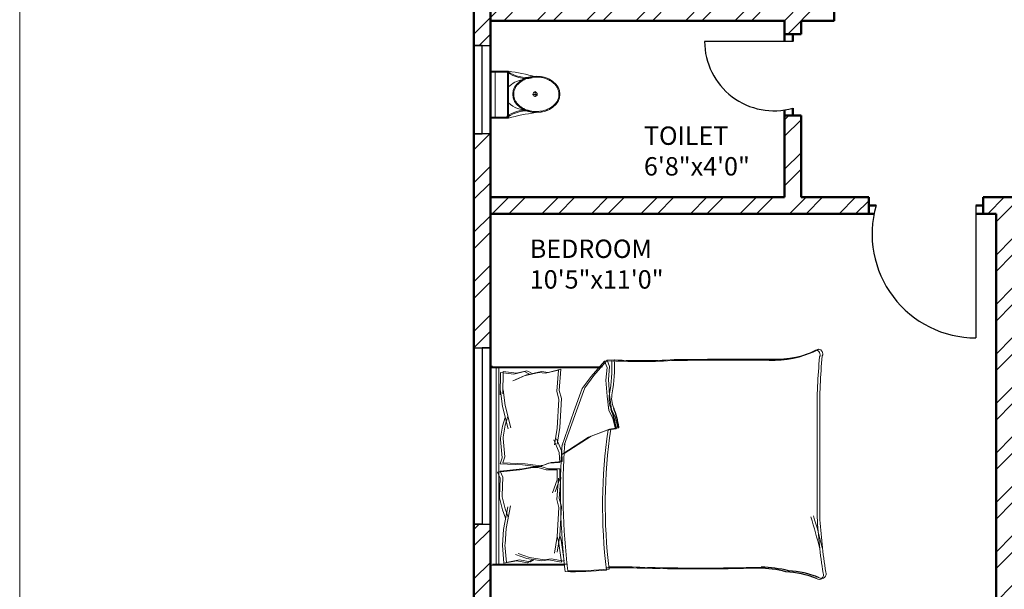
# Model space of a CAD drawing. Units: inches. Extents: x 1901 to 2863, y 888 to 2433.
# Tile 50 of 91: x 1901 to 2169, y 1847 to 2002. Entities that reach past the tile are written whole.
import ezdxf

# ---------------------------------------------------------------- set-up
doc = ezdxf.new("R2010")
doc.units = ezdxf.units.IN
for name, color, linetype, lineweight in [('A-AREA-IDEN', 7, 'Continuous', 18), ('A-DOOR', 4, 'Continuous', 25), ('A-FLOR-FIXT', 9, 'Continuous', 18), ('A-FURN', 8, 'Continuous', 18), ('A-GLAZ', 3, 'Continuous', 25), ('A-WALL', 7, 'Continuous', 50), ('A-WALL-PATT', 8, 'Continuous', 13)]:
    doc.layers.add(name, color=color, linetype=linetype, lineweight=lineweight)
doc.styles.get("Standard").update_dxf_attribs({"font": 'arial.ttf'})

# ---------------------------------------------------------------- blocks, each defined once
blk = doc.blocks.new('A$C31115884')
for p, q in [((283, 498), (223, 498)), ((258, 466), (258, 523)), ((0, 200), (0, 0)), ((520, 200), (0, 200)), ((10, 190), (10, 10)), ((510, 190), (10, 190)), ((510, 10), (510, 190)), ((520, 0), (520, 200)), ((510, 54), (0, 54)), ((10, 10), (510, 10)), ((0, 0), (520, 0))]:
    blk.add_line(p, q)
blk.add_circle((256, 496), 23.6)
for centre, radius, start, end in [((2778, -205), 2807, 165.4549, 171.7133), ((-295, 403), 365, 324.2091, 9.3499), ((-295, 403), 375, 324.2091, 9.3499), ((806, 403), 365, 170.6501, 215.7909), ((3237, 905), 2807, 188.2867, 194.5451), ((384, 406), 293, 190.2774, 224.1564), ((139, 406), 293, 315.8436, 2.6563), ((806, 403), 375, 179.2036, 215.7909)]:
    blk.add_arc(centre, radius, start, end)
blk.add_ellipse((256, 510), major_axis=(0, -261), ratio=0.772727)
blk.add_open_spline([(256, 259), (263, 259), (270, 260), (288, 262), (299, 265), (320, 273), (330, 278), (350, 291), (360, 299), (378, 316), (386, 326), (402, 347), (409, 358), (421, 383), (427, 395), (436, 422), (440, 436), (445, 465), (447, 480), (448, 509), (448, 524), (445, 553), (443, 568), (436, 596), (432, 610), (422, 636), (416, 649), (402, 672), (395, 683), (379, 703), (370, 712), (351, 728), (341, 735), (321, 746), (310, 751), (289, 757), (278, 759), (256, 761), (245, 761), (223, 757), (212, 754), (191, 746), (181, 741), (161, 728), (151, 720), (133, 703), (125, 693), (110, 672), (103, 660), (90, 636), (85, 623), (76, 596), (72, 582), (67, 553), (66, 538), (64, 509), (65, 494), (68, 465), (70, 450), (77, 422), (81, 408), (91, 382), (97, 370), (111, 346), (118, 335), (135, 316), (144, 307), (162, 291), (172, 284), (193, 273), (203, 269), (225, 262), (236, 260), (250, 259), (253, 259), (256, 259)], degree=3, knots=[0, 0, 0, 0, 0.110105, 0.110105, 0.285049, 0.285049, 0.459994, 0.459994, 0.634938, 0.634938, 0.809882, 0.809882, 0.984827, 0.984827, 1.159771, 1.159771, 1.334715, 1.334715, 1.50966, 1.50966, 1.684604, 1.684604, 1.859549, 1.859549, 2.034493, 2.034493, 2.209437, 2.209437, 2.384382, 2.384382, 2.559326, 2.559326, 2.73427, 2.73427, 2.909215, 2.909215, 3.084159, 3.084159, 3.259103, 3.259103, 3.434048, 3.434048, 3.608992, 3.608992, 3.783936, 3.783936, 3.958881, 3.958881, 4.133825, 4.133825, 4.30877, 4.30877, 4.483714, 4.483714, 4.658658, 4.658658, 4.833603, 4.833603, 5.008547, 5.008547, 5.183491, 5.183491, 5.358436, 5.358436, 5.53338, 5.53338, 5.708324, 5.708324, 5.883269, 5.883269, 6.058213, 6.058213, 6.233158, 6.233158, 6.283185, 6.283185, 6.283185, 6.283185])
blk = doc.blocks.new('WIN-48')
for p, q in [((0, 2.25), (0, 4.5)), ((0, 4.5), (0, 0)), ((48, 4.5), (48, 0)), ((48, 2.25), (0, 2.25)), ((48, 0), (48, 2.25))]:
    blk.add_line(p, q)
blk = doc.blocks.new('WIN-24-3')
for p, q in [((0, 0), (0, 4.5)), ((0, 4.5), (0, 2.25)), ((24, 2.25), (24, 4.5)), ((24, 4.5), (24, 0)), ((0, 2.25), (24, 2.25))]:
    blk.add_line(p, q)
blk = doc.blocks.new('DOOR-28')
blk.add_line((28.27, 35.98), (28.27, -0.02))
blk.add_arc((28.27, 28.24), 28.25, 164.0861, 270)

msp = doc.modelspace()

# ---------------------------------------------------------------- hatches: boundary and pattern name
at = {"layer": 'A-WALL-PATT'}
h = msp.add_hatch(dxfattribs=at)
h.set_pattern_fill('ANSI32', color=256)
h.paths.add_polyline_path([(2192.5, 2274.13), (2141.26, 2274.13), (2141.26, 2269.63), (2192.5, 2269.63)])
h.paths.add_polyline_path([(2259.93, 2274.13), (2216.5, 2274.13), (2216.5, 2269.63), (2255.43, 2269.63), (2255.43, 2214.63), (2250.81, 2214.63), (2250.81, 2210.13), (2259.93, 2210.13), (2259.93, 2215.13), (2271.76, 2215.13), (2271.76, 2217.38), (2271.76, 2219.63), (2259.93, 2219.63)])
h.paths.add_polyline_path([(2171.43, 2269.63), (2166.93, 2269.63), (2166.93, 2219.63), (2121.24, 2219.63), (2121.24, 2215.13), (2166.93, 2215.13), (2166.93, 2083.13), (2161.81, 2083.13), (2161.81, 2078.63), (2171.43, 2078.63), (2177, 2078.63), (2177, 2080.88), (2177, 2083.13), (2171.43, 2083.13), (2171.43, 2210.13), (2230.91, 2210.13), (2230.91, 2212.38), (2230.91, 2214.63), (2171.43, 2214.63)])
h.paths.add_polyline_path([(2117.26, 2274.13), (2089.43, 2274.13), (2089.43, 2219.63), (2081.14, 2219.63), (2081.14, 2215.13), (2089.43, 2215.13), (2098, 2215.13), (2098, 2217.38), (2098, 2219.63), (2093.93, 2219.63), (2093.93, 2269.63), (2117.26, 2269.63), (2117.26, 2271.88)])
h.paths.add_polyline_path([(2343.43, 2219.63), (2329.29, 2219.63), (2329.29, 2215.13), (2338.93, 2215.13), (2338.93, 2184.74), (2343.43, 2184.74)])
h.paths.add_polyline_path([(2338.93, 2083.13), (2329.29, 2083.13), (2208.97, 2083.13), (2208.97, 2078.63), (2338.93, 2078.63)])
h.paths.add_polyline_path([(2343.43, 2136.74), (2338.93, 2136.74), (2338.93, 1872.63), (2343.43, 1872.63)])
h.paths.add_polyline_path([(2343.43, 1863.63), (2397.68, 1863.63), (2397.68, 1821.63), (2384.14, 1821.63), (2384.14, 1812.63), (2418.33, 1812.63), (2418.33, 1817.13), (2418.33, 1821.63), (2406.68, 1821.63), (2406.68, 1863.63), (2459.5, 1863.63), (2459.5, 1821.63), (2447.14, 1821.63), (2447.14, 1812.63), (2459.5, 1812.63), (2468.5, 1812.63), (2468.5, 1872.63), (2394.43, 1872.63), (2334.43, 1872.63), (2334.43, 1812.63), (2343.43, 1812.63), (2353.25, 1812.63), (2353.25, 1821.63), (2343.43, 1821.63)])
h.paths.add_polyline_path([(2510.01, 1872.63), (2468.5, 1872.63), (2468.5, 1868.13), (2510.01, 1868.13)])
h.paths.add_polyline_path([(2514.01, 1817.13), (2468.5, 1817.13), (2468.5, 1812.63), (2482.11, 1812.63), (2482.11, 1800.61), (2486.61, 1800.61), (2486.61, 1812.63), (2514.01, 1812.63)])
h.paths.add_polyline_path([(2299.25, 1814.88), (2299.25, 1817.13), (2295.93, 1817.13), (2295.93, 1854.17), (2293.68, 1854.17), (2291.43, 1854.17), (2291.43, 1817.13), (2266.11, 1817.13), (2266.11, 1812.63), (2299.25, 1812.63)])
h.paths.add_polyline_path([(2218.11, 1817.13), (2206.46, 1817.13), (2171.43, 1817.13), (2171.43, 1949.13), (2190.1, 1949.13), (2190.1, 1953.63), (2163.47, 1953.63), (2163.47, 1949.13), (2166.93, 1949.13), (2166.93, 1817.13), (2114.3, 1817.13), (2114.3, 1812.63), (2218.11, 1812.63)])
h.paths.add_polyline_path([(2029.43, 1970.92), (2024.93, 1970.92), (2024.93, 1912.72), (2029.43, 1912.72)])
h.paths.add_polyline_path([(2132.3, 1953.63), (2113.93, 1953.63), (2113.93, 1975.89), (2111.68, 1975.89), (2109.43, 1975.89), (2109.43, 1953.63), (2029.43, 1953.63), (2029.43, 1949.13), (2132.3, 1949.13)])
h.paths.add_polyline_path([(2029.43, 1853.61), (2029.31, 1853.61), (2029.31, 1853.61), (2029.43, 1853.61), (2029.43, 1864.72), (2024.93, 1864.72), (2024.93, 1812.63), (2066.3, 1812.63), (2066.3, 1814.88), (2066.3, 1817.13), (2029.43, 1817.13)])
h.paths.add_polyline_path([(2122.93, 2010.09), (2120.68, 2010.09), (2118.43, 2010.09), (2118.43, 2006.13), (2029.43, 2006.13), (2029.43, 2001.63), (2109.43, 2001.63), (2109.43, 1998.04), (2113.93, 1998.04), (2113.93, 2001.63), (2122.93, 2001.63)])
h.paths.add_polyline_path([(2029.43, 2031.38), (2024.93, 2031.38), (2024.93, 1994.92), (2027.18, 1994.92), (2029.43, 1994.92)])
h.paths.add_polyline_path([(2029.43, 2136.74), (2024.93, 2136.74), (2024.93, 2067.38), (2027.18, 2067.38), (2029.43, 2067.38)])
h.paths.add_polyline_path([(2125.62, 2083.13), (2029.43, 2083.13), (2029.43, 2078.63), (2118.43, 2078.63), (2118.43, 2030.71), (2122.93, 2030.71), (2122.93, 2078.63), (2125.62, 2078.63)])
h.paths.add_polyline_path([(2029.43, 2215.13), (2040.47, 2215.13), (2040.47, 2217.38), (2040.47, 2219.63), (2024.93, 2219.63), (2024.93, 2184.74), (2029.43, 2184.74), (2029.43, 2187.78)])
h.paths.add_polyline_path([(2686.43, 2274.13), (2659.28, 2274.13), (2659.28, 2269.63), (2681.93, 2269.63), (2681.93, 2219.63), (2676.82, 2219.63), (2676.82, 2215.13), (2681.93, 2215.13), (2697.01, 2215.13), (2697.01, 2217.38), (2697.01, 2219.63), (2686.43, 2219.63)])
h.paths.add_polyline_path([(2609.93, 2269.63), (2635.28, 2269.63), (2635.28, 2274.13), (2571.43, 2274.13), (2571.43, 2269.63), (2605.43, 2269.63), (2605.43, 2214.63), (2549.1, 2214.63), (2549.1, 2210.13), (2605.43, 2210.13), (2605.43, 2083.13), (2601.01, 2083.13), (2601.01, 2080.88), (2601.01, 2078.63), (2609.93, 2078.63), (2616.16, 2078.63), (2616.16, 2080.88), (2616.16, 2083.13), (2609.93, 2083.13), (2609.93, 2215.13), (2651.46, 2215.13), (2651.46, 2217.38), (2651.46, 2219.63), (2609.93, 2219.63)])
h.paths.add_polyline_path([(2521.43, 2269.63), (2547.43, 2269.63), (2547.43, 2271.88), (2547.43, 2274.13), (2516.93, 2274.13), (2516.93, 2219.63), (2506.41, 2219.63), (2506.41, 2215.13), (2516.93, 2215.13), (2516.93, 2210.13), (2525.4, 2210.13), (2525.4, 2212.38), (2525.4, 2214.63), (2521.43, 2214.63)])
h.paths.add_polyline_path([(2456.01, 2219.63), (2439.43, 2219.63), (2439.43, 2187.89), (2443.93, 2187.89), (2443.93, 2215.13), (2456.01, 2215.13)])
h.paths.add_polyline_path([(2752.93, 2219.63), (2739.48, 2219.63), (2739.48, 2215.13), (2748.43, 2215.13), (2748.43, 2187.89), (2752.93, 2187.89)])
h.paths.add_polyline_path([(2752.93, 2139.89), (2748.43, 2139.89), (2748.43, 2083.13), (2648.42, 2083.13), (2648.42, 2078.63), (2654.93, 2078.63), (2654.93, 2039.44), (2659.43, 2039.44), (2659.43, 2078.63), (2748.43, 2078.63), (2748.43, 2063.43), (2752.93, 2063.43)])
h.paths.add_polyline_path([(2752.93, 2010.63), (2659.43, 2010.63), (2659.43, 2015.65), (2654.93, 2015.65), (2654.93, 2010.63), (2605.43, 2010.63), (2605.43, 1920.97), (2609.93, 1920.97), (2609.93, 2006.13), (2748.43, 2006.13), (2748.43, 1982.47), (2752.93, 1982.47)])
h.paths.add_polyline_path([(2752.93, 2027.43), (2748.43, 2027.43), (2748.43, 2010.63), (2752.93, 2010.63)])
h.paths.add_polyline_path([(2748.43, 1886.13), (2609.93, 1886.13), (2609.93, 1889.72), (2605.43, 1889.72), (2605.43, 1861.26), (2609.93, 1861.26), (2609.93, 1881.63), (2748.43, 1881.63)])
h.paths.add_polyline_path([(2456.86, 2228.83), (2498.4, 2228.83), (2498.4, 2247.49), (2456.86, 2247.49)], flags=9)
h.paths.add_polyline_path([(2038.6, 2237.42), (2080.17, 2237.42), (2080.17, 2256.08), (2038.6, 2256.08)], flags=9)
h.paths.add_polyline_path([(2292.01, 1062.39), (2539.93, 1062.39), (2539.93, 1099.49), (2292.01, 1099.49)], flags=9)
h.paths.add_polyline_path([(2424.91, 1832.25), (2448.51, 1832.25), (2448.51, 1846.68), (2424.91, 1846.68)], flags=25)
h.paths.add_polyline_path([(2359.08, 1832.25), (2382.68, 1832.25), (2382.68, 1846.68), (2359.08, 1846.68)], flags=25)
h.paths.add_polyline_path([(2352.9, 1684.8), (2367.54, 1684.8), (2367.54, 1697.17), (2352.9, 1697.17)], flags=9)
h.paths.add_polyline_path([(2079.29, 1755.83), (2169.02, 1755.83), (2169.02, 1774.37), (2079.29, 1774.37)], flags=9)
h.paths.add_polyline_path([(2404.09, 1373.86), (2404.09, 1463.59), (2385.54, 1463.59), (2385.54, 1373.86)], flags=9)
h.paths.add_polyline_path([(2268.09, 2236.37), (2309.64, 2236.37), (2309.64, 2255.03), (2268.09, 2255.03)], flags=9)
h.paths.add_polyline_path([(2575.96, 1700.95), (2665.7, 1700.95), (2665.7, 1719.5), (2575.96, 1719.5)], flags=9)
h.paths.add_polyline_path([(2302.96, 1878.47), (2329.52, 1878.47), (2329.52, 1888.78), (2302.96, 1888.78)], flags=9)
h.paths.add_polyline_path([(2097.42, 2240.58), (2126.57, 2240.58), (2126.57, 2259.23), (2097.42, 2259.23)], flags=9)
h.paths.add_polyline_path([(2208.72, 2246.12), (2237.88, 2246.12), (2237.88, 2264.78), (2208.72, 2264.78)], flags=9)
h.paths.add_polyline_path([(2038.15, 1925.96), (2076.99, 1925.96), (2076.99, 1944.62), (2038.15, 1944.62)], flags=9)
h.paths.add_polyline_path([(2239.14, 1926.67), (2288.46, 1926.67), (2288.46, 1945.33), (2239.14, 1945.33)], flags=9)
h.paths.add_polyline_path([(2175.43, 2007.33), (2212.36, 2007.33), (2212.36, 2025.99), (2175.43, 2025.99)], flags=9)
h.paths.add_polyline_path([(2225.03, 2091.79), (2263.87, 2091.79), (2263.87, 2110.45), (2225.03, 2110.45)], flags=9)
h.paths.add_polyline_path([(2035.4, 2098.48), (2074.24, 2098.48), (2074.24, 2117.14), (2035.4, 2117.14)], flags=9)
h.paths.add_polyline_path([(2050.1, 2029.21), (2083.26, 2029.21), (2083.26, 2047.87), (2050.1, 2047.87)], flags=9)
h.paths.add_polyline_path([(2069.68, 1956.72), (2098.83, 1956.72), (2098.83, 1975.38), (2069.68, 1975.38)], flags=25)
h.paths.add_polyline_path([(2328.62, 1753.34), (2361.66, 1753.34), (2361.66, 1771.99), (2328.62, 1771.99)], flags=9)
h.paths.add_polyline_path([(2395.16, 2060.89), (2395.16, 2140.65), (2378.68, 2140.65), (2378.68, 2060.89)], flags=9)
h.paths.add_polyline_path([(2463.73, 2059.02), (2492.89, 2059.02), (2492.89, 2077.68), (2463.73, 2077.68)], flags=9)
h.paths.add_polyline_path([(2458.03, 2181.54), (2496.87, 2181.54), (2496.87, 2200.19), (2458.03, 2200.19)], flags=9)
h.paths.add_polyline_path([(2527.58, 2243.07), (2556.73, 2243.07), (2556.73, 2261.73), (2527.58, 2261.73)], flags=9)
h.paths.add_polyline_path([(2694.46, 2232.77), (2736.03, 2232.77), (2736.03, 2251.42), (2694.46, 2251.42)], flags=9)
h.paths.add_polyline_path([(2637.82, 2249.22), (2666.98, 2249.22), (2666.98, 2267.88), (2637.82, 2267.88)], flags=9)
h.paths.add_polyline_path([(2623.69, 2183.54), (2662.53, 2183.54), (2662.53, 2202.2), (2623.69, 2202.2)], flags=9)
h.paths.add_polyline_path([(2691.97, 2021.5), (2725.12, 2021.5), (2725.12, 2040.16), (2691.97, 2040.16)], flags=9)
h.paths.add_polyline_path([(2621.04, 1975.91), (2662.34, 1975.91), (2662.34, 1994.57), (2621.04, 1994.57)], flags=25)
h.paths.add_polyline_path([(2479.03, 1927.62), (2519.84, 1927.62), (2519.84, 1946.28), (2479.03, 1946.28)], flags=9)
h.paths.add_polyline_path([(2670.94, 1849.08), (2716.01, 1849.08), (2716.01, 1867.73), (2670.94, 1867.73)], flags=9)
h.paths.add_polyline_path([(2523.61, 1782.96), (2550.17, 1782.96), (2550.17, 1793.26), (2523.61, 1793.26)], flags=9)
h.paths.add_polyline_path([(2450.84, 1207.33), (2492.39, 1207.33), (2492.39, 1225.99), (2450.84, 1225.99)], flags=9)
h.paths.add_polyline_path([(2527.75, 1203.84), (2556.91, 1203.84), (2556.91, 1222.5), (2527.75, 1222.5)], flags=9)
h.paths.add_polyline_path([(2639.11, 1207.2), (2668.27, 1207.2), (2668.27, 1225.86), (2639.11, 1225.86)], flags=9)
h.paths.add_polyline_path([(2692.59, 1218.97), (2734.17, 1218.97), (2734.17, 1237.62), (2692.59, 1237.62)], flags=9)
h.paths.add_polyline_path([(2669.27, 1366.33), (2708.11, 1366.33), (2708.11, 1384.99), (2669.27, 1384.99)], flags=9)
h.paths.add_polyline_path([(2463.31, 1358.03), (2502.15, 1358.03), (2502.15, 1376.69), (2463.31, 1376.69)], flags=9)
h.paths.add_polyline_path([(2494.72, 1449.96), (2531.65, 1449.96), (2531.65, 1468.62), (2494.72, 1468.62)], flags=9)
h.paths.add_polyline_path([(2675.57, 1422.16), (2708.72, 1422.16), (2708.72, 1440.81), (2675.57, 1440.81)], flags=9)
h.paths.add_polyline_path([(2685.63, 1493.89), (2714.79, 1493.89), (2714.79, 1512.55), (2685.63, 1512.55)], flags=9)
h.paths.add_polyline_path([(2686.8, 1529.91), (2725.65, 1529.91), (2725.65, 1548.57), (2686.8, 1548.57)], flags=9)
h.paths.add_polyline_path([(2503.65, 1537.99), (2552.97, 1537.99), (2552.97, 1556.65), (2503.65, 1556.65)], flags=9)
h.paths.add_polyline_path([(2291.71, 1643.5), (2318.28, 1643.5), (2318.28, 1653.81), (2291.71, 1653.81)], flags=9)
h.paths.add_polyline_path([(2450.63, 1610.52), (2477.19, 1610.52), (2477.19, 1620.82), (2450.63, 1620.82)], flags=9)
h.paths.add_polyline_path([(2359.99, 1551.81), (2422.25, 1551.81), (2422.25, 1562.12), (2359.99, 1562.12)], flags=9)
h.paths.add_polyline_path([(2280.11, 1249.01), (2321.65, 1249.01), (2321.65, 1267.66), (2280.11, 1267.66)], flags=9)
h.paths.add_polyline_path([(2164.06, 1274.23), (2193.22, 1274.23), (2193.22, 1292.89), (2164.06, 1292.89)], flags=9)
h.paths.add_polyline_path([(2118.21, 1277.69), (2151.25, 1277.69), (2151.25, 1296.35), (2118.21, 1296.35)], flags=9)
h.paths.add_polyline_path([(2031.95, 1268.53), (2073.52, 1268.53), (2073.52, 1287.19), (2031.95, 1287.19)], flags=9)
h.paths.add_polyline_path([(2050.2, 1409.08), (2089.04, 1409.08), (2089.04, 1427.74), (2050.2, 1427.74)], flags=9)
h.paths.add_polyline_path([(2243.74, 1421.03), (2282.58, 1421.03), (2282.58, 1439.69), (2243.74, 1439.69)], flags=9)
h.paths.add_polyline_path([(2190.75, 1509.77), (2231.56, 1509.77), (2231.56, 1528.43), (2190.75, 1528.43)], flags=9)
h.paths.add_polyline_path([(2058.39, 1475.42), (2091.55, 1475.42), (2091.55, 1494.07), (2058.39, 1494.07)], flags=9)
h.paths.add_polyline_path([(2062.45, 1553.09), (2091.6, 1553.09), (2091.6, 1571.75), (2062.45, 1571.75)], flags=9)
h.paths.add_polyline_path([(2219.52, 1590.37), (2266.15, 1590.37), (2266.15, 1609.02), (2219.52, 1609.02)], flags=9)
h.paths.add_polyline_path([(2041.07, 1584.19), (2079.91, 1584.19), (2079.91, 1602.85), (2041.07, 1602.85)], flags=9)
h = msp.add_hatch(dxfattribs=at)
h.set_pattern_fill('ANSI32', color=256)
h.paths.add_polyline_path([(2443.93, 2139.89), (2439.43, 2139.89), (2439.43, 2069.35), (2441.68, 2069.35), (2443.93, 2069.35), (2443.93, 2078.63), (2521.93, 2078.63), (2521.93, 2075.07), (2524.18, 2075.07), (2526.43, 2075.07), (2526.43, 2078.63), (2571.75, 2078.63), (2571.75, 2080.88), (2571.75, 2083.13), (2443.93, 2083.13)])
h.paths.add_polyline_path([(2526.43, 2054.63), (2524.18, 2054.63), (2521.93, 2054.63), (2521.93, 2030.63), (2443.93, 2030.63), (2443.93, 2045.35), (2439.43, 2045.35), (2439.43, 1983.87), (2443.93, 1983.87), (2443.93, 2026.13), (2521.93, 2026.13), (2526.43, 2026.13)])
h.paths.add_polyline_path([(2443.93, 1923.87), (2439.43, 1923.87), (2439.43, 1872.63), (2443.93, 1872.63)])
h.paths.add_polyline_path([(2636.23, 1766.13), (2609.93, 1766.13), (2609.93, 1779.79), (2605.43, 1779.79), (2605.43, 1766.13), (2486.61, 1766.13), (2486.61, 1770.67), (2482.11, 1770.67), (2482.11, 1766.13), (2482.11, 1761.63), (2636.23, 1761.63), (2636.23, 1763.88)])
h.paths.add_polyline_path([(2519.54, 1663.38), (2519.54, 1665.63), (2494.93, 1665.63), (2481.83, 1665.63), (2481.83, 1663.38), (2481.83, 1661.13), (2490.43, 1661.13), (2490.43, 1640.16), (2494.93, 1640.16), (2494.93, 1661.13), (2519.54, 1661.13)])
h.paths.add_polyline_path([(2443.93, 1712.13), (2443.93, 1716.63), (2414.46, 1716.63), (2414.46, 1712.13), (2439.43, 1712.13), (2439.43, 1545.51), (2443.93, 1545.51), (2443.93, 1661.13), (2448.47, 1661.13), (2448.47, 1665.63), (2443.93, 1665.63)])
h.paths.add_polyline_path([(2343.43, 1712.13), (2365.52, 1712.13), (2365.52, 1714.38), (2365.52, 1716.63), (2333.87, 1716.63), (2333.87, 1714.38), (2333.87, 1712.13), (2338.93, 1712.13), (2338.93, 1575.63), (2338.93, 1545.51), (2343.43, 1545.51), (2343.43, 1547.51), (2343.43, 1580.13)])
h.paths.add_polyline_path([(2752.93, 1665.63), (2579.54, 1665.63), (2579.54, 1661.13), (2615.93, 1661.13), (2615.93, 1529.13), (2598.93, 1529.13), (2598.93, 1524.63), (2623.13, 1524.63), (2623.13, 1526.88), (2623.13, 1529.13), (2620.43, 1529.13), (2620.43, 1661.13), (2748.43, 1661.13), (2748.43, 1633.5), (2752.93, 1633.5)])
h.paths.add_polyline_path([(2752.93, 1419.93), (2748.43, 1419.93), (2748.43, 1400.13), (2659.43, 1400.13), (2659.43, 1444.33), (2657.18, 1444.33), (2654.93, 1444.33), (2654.93, 1400.13), (2643.65, 1400.13), (2643.65, 1395.63), (2748.43, 1395.63), (2748.43, 1364.04), (2752.93, 1364.04)])
h.paths.add_polyline_path([(2752.93, 1492.88), (2748.43, 1492.88), (2748.43, 1476.63), (2667.43, 1476.63), (2667.43, 1479.71), (2665.18, 1479.71), (2662.93, 1479.71), (2662.93, 1476.63), (2654.93, 1476.63), (2654.93, 1469.54), (2659.43, 1469.54), (2659.43, 1472.13), (2748.43, 1472.13), (2748.43, 1455.93), (2752.93, 1455.93)])
h.paths.add_polyline_path([(2752.93, 1304.04), (2748.43, 1304.04), (2748.43, 1263.63), (2738.66, 1263.63), (2738.66, 1259.13), (2752.93, 1259.13)])
h.paths.add_polyline_path([(2685.93, 1259.13), (2695.49, 1259.13), (2695.49, 1261.38), (2695.49, 1263.63), (2677.84, 1263.63), (2677.84, 1261.38), (2677.84, 1259.13), (2681.43, 1259.13), (2681.43, 1203.63), (2653.28, 1203.63), (2653.28, 1199.13), (2685.93, 1199.13), (2685.93, 1203.63)])
h.paths.add_polyline_path([(2609.43, 1395.63), (2611.85, 1395.63), (2611.85, 1400.13), (2598.89, 1400.13), (2598.89, 1397.88), (2598.89, 1395.63), (2604.93, 1395.63), (2604.93, 1268.13), (2554.73, 1268.13), (2554.73, 1265.88), (2554.73, 1263.63), (2604.93, 1263.63), (2604.93, 1203.63), (2571.31, 1203.63), (2571.31, 1199.13), (2604.93, 1199.13), (2629.28, 1199.13), (2629.28, 1201.38), (2629.28, 1203.63), (2609.43, 1203.63), (2609.43, 1258.63), (2609.43, 1259.13), (2654.8, 1259.13), (2654.8, 1263.63), (2609.43, 1263.63)])
h.paths.add_polyline_path([(2443.93, 1304.04), (2439.43, 1304.04), (2439.43, 1259.13), (2443.93, 1259.13), (2456.16, 1259.13), (2456.16, 1261.38), (2456.16, 1263.63), (2443.93, 1263.63)])
h.paths.add_polyline_path([(2525.43, 1263.63), (2531.78, 1263.63), (2531.78, 1268.13), (2520.93, 1268.13), (2520.93, 1263.63), (2511.41, 1263.63), (2511.41, 1259.13), (2520.93, 1259.13), (2520.93, 1199.13), (2547.31, 1199.13), (2547.31, 1201.38), (2547.31, 1203.63), (2525.43, 1203.63)])
h.paths.add_polyline_path([(2443.93, 1434.84), (2439.43, 1434.84), (2439.43, 1364.04), (2441.68, 1364.04), (2443.93, 1364.04)])
h.paths.add_polyline_path([(2567.13, 1400.13), (2443.93, 1400.13), (2443.93, 1395.63), (2567.13, 1395.63)])
h.paths.add_polyline_path([(2443.93, 1545.51), (2439.43, 1545.51), (2439.43, 1494.84), (2443.93, 1494.84)])
h.paths.add_polyline_path([(2494.93, 1553.35), (2492.68, 1553.35), (2490.43, 1553.35), (2490.43, 1524.63), (2494.93, 1524.63), (2525.94, 1524.63), (2525.94, 1526.88), (2525.94, 1529.13), (2494.93, 1529.13)])
h.paths.add_polyline_path([(2752.93, 1573.5), (2748.43, 1573.5), (2748.43, 1529.13), (2657.76, 1529.13), (2657.76, 1524.63), (2662.93, 1524.63), (2662.93, 1498.63), (2667.43, 1498.63), (2667.43, 1524.63), (2748.43, 1524.63), (2748.43, 1516.88), (2752.93, 1516.88)])
h.paths.add_polyline_path([(2038.6, 2237.42), (2080.17, 2237.42), (2080.17, 2256.08), (2038.6, 2256.08)], flags=9)
h.paths.add_polyline_path([(2292.01, 1062.39), (2539.93, 1062.39), (2539.93, 1099.49), (2292.01, 1099.49)], flags=9)
h.paths.add_polyline_path([(2424.91, 1832.25), (2448.51, 1832.25), (2448.51, 1846.68), (2424.91, 1846.68)], flags=9)
h.paths.add_polyline_path([(2359.08, 1832.25), (2382.68, 1832.25), (2382.68, 1846.68), (2359.08, 1846.68)], flags=9)
h.paths.add_polyline_path([(2352.9, 1684.8), (2367.54, 1684.8), (2367.54, 1697.17), (2352.9, 1697.17)], flags=9)
h.paths.add_polyline_path([(2079.29, 1755.83), (2169.02, 1755.83), (2169.02, 1774.37), (2079.29, 1774.37)], flags=9)
h.paths.add_polyline_path([(2404.09, 1373.86), (2404.09, 1463.59), (2385.54, 1463.59), (2385.54, 1373.86)], flags=9)
h.paths.add_polyline_path([(2268.09, 2236.37), (2309.64, 2236.37), (2309.64, 2255.03), (2268.09, 2255.03)], flags=9)
h.paths.add_polyline_path([(2575.96, 1700.95), (2665.7, 1700.95), (2665.7, 1719.5), (2575.96, 1719.5)], flags=9)
h.paths.add_polyline_path([(2302.96, 1878.47), (2329.52, 1878.47), (2329.52, 1888.78), (2302.96, 1888.78)], flags=9)
h.paths.add_polyline_path([(2097.42, 2240.58), (2126.57, 2240.58), (2126.57, 2259.23), (2097.42, 2259.23)], flags=9)
h.paths.add_polyline_path([(2208.72, 2246.12), (2237.88, 2246.12), (2237.88, 2264.78), (2208.72, 2264.78)], flags=9)
h.paths.add_polyline_path([(2038.15, 1925.96), (2076.99, 1925.96), (2076.99, 1944.62), (2038.15, 1944.62)], flags=9)
h.paths.add_polyline_path([(2239.14, 1926.67), (2288.46, 1926.67), (2288.46, 1945.33), (2239.14, 1945.33)], flags=9)
h.paths.add_polyline_path([(2175.43, 2007.33), (2212.36, 2007.33), (2212.36, 2025.99), (2175.43, 2025.99)], flags=9)
h.paths.add_polyline_path([(2225.03, 2091.79), (2263.87, 2091.79), (2263.87, 2110.45), (2225.03, 2110.45)], flags=9)
h.paths.add_polyline_path([(2035.4, 2098.48), (2074.24, 2098.48), (2074.24, 2117.14), (2035.4, 2117.14)], flags=9)
h.paths.add_polyline_path([(2050.1, 2029.21), (2083.26, 2029.21), (2083.26, 2047.87), (2050.1, 2047.87)], flags=9)
h.paths.add_polyline_path([(2069.68, 1956.72), (2098.83, 1956.72), (2098.83, 1975.38), (2069.68, 1975.38)], flags=9)
h.paths.add_polyline_path([(2328.62, 1753.34), (2361.66, 1753.34), (2361.66, 1771.99), (2328.62, 1771.99)], flags=9)
h.paths.add_polyline_path([(2395.16, 2060.89), (2395.16, 2140.65), (2378.68, 2140.65), (2378.68, 2060.89)], flags=9)
h.paths.add_polyline_path([(2463.73, 2059.02), (2492.89, 2059.02), (2492.89, 2077.68), (2463.73, 2077.68)], flags=9)
h.paths.add_polyline_path([(2458.03, 2181.54), (2496.87, 2181.54), (2496.87, 2200.19), (2458.03, 2200.19)], flags=9)
h.paths.add_polyline_path([(2456.86, 2228.83), (2498.4, 2228.83), (2498.4, 2247.49), (2456.86, 2247.49)], flags=9)
h.paths.add_polyline_path([(2527.58, 2243.07), (2556.73, 2243.07), (2556.73, 2261.73), (2527.58, 2261.73)], flags=9)
h.paths.add_polyline_path([(2694.46, 2232.77), (2736.03, 2232.77), (2736.03, 2251.42), (2694.46, 2251.42)], flags=9)
h.paths.add_polyline_path([(2637.82, 2249.22), (2666.98, 2249.22), (2666.98, 2267.88), (2637.82, 2267.88)], flags=9)
h.paths.add_polyline_path([(2623.69, 2183.54), (2662.53, 2183.54), (2662.53, 2202.2), (2623.69, 2202.2)], flags=9)
h.paths.add_polyline_path([(2691.97, 2021.5), (2725.12, 2021.5), (2725.12, 2040.16), (2691.97, 2040.16)], flags=9)
h.paths.add_polyline_path([(2621.04, 1975.91), (2662.34, 1975.91), (2662.34, 1994.57), (2621.04, 1994.57)], flags=9)
h.paths.add_polyline_path([(2479.03, 1927.62), (2519.84, 1927.62), (2519.84, 1946.28), (2479.03, 1946.28)], flags=9)
h.paths.add_polyline_path([(2670.94, 1849.08), (2716.01, 1849.08), (2716.01, 1867.73), (2670.94, 1867.73)], flags=9)
h.paths.add_polyline_path([(2523.61, 1782.96), (2550.17, 1782.96), (2550.17, 1793.26), (2523.61, 1793.26)], flags=9)
h.paths.add_polyline_path([(2450.84, 1207.33), (2492.39, 1207.33), (2492.39, 1225.99), (2450.84, 1225.99)], flags=9)
h.paths.add_polyline_path([(2527.75, 1203.84), (2556.91, 1203.84), (2556.91, 1222.5), (2527.75, 1222.5)], flags=9)
h.paths.add_polyline_path([(2639.11, 1207.2), (2668.27, 1207.2), (2668.27, 1225.86), (2639.11, 1225.86)], flags=9)
h.paths.add_polyline_path([(2692.59, 1218.97), (2734.17, 1218.97), (2734.17, 1237.62), (2692.59, 1237.62)], flags=9)
h.paths.add_polyline_path([(2669.27, 1366.33), (2708.11, 1366.33), (2708.11, 1384.99), (2669.27, 1384.99)], flags=25)
h.paths.add_polyline_path([(2463.31, 1358.03), (2502.15, 1358.03), (2502.15, 1376.69), (2463.31, 1376.69)], flags=9)
h.paths.add_polyline_path([(2494.72, 1449.96), (2531.65, 1449.96), (2531.65, 1468.62), (2494.72, 1468.62)], flags=9)
h.paths.add_polyline_path([(2675.57, 1422.16), (2708.72, 1422.16), (2708.72, 1440.81), (2675.57, 1440.81)], flags=25)
h.paths.add_polyline_path([(2685.63, 1493.89), (2714.79, 1493.89), (2714.79, 1512.55), (2685.63, 1512.55)], flags=9)
h.paths.add_polyline_path([(2686.8, 1529.91), (2725.65, 1529.91), (2725.65, 1548.57), (2686.8, 1548.57)], flags=25)
h.paths.add_polyline_path([(2503.65, 1537.99), (2552.97, 1537.99), (2552.97, 1556.65), (2503.65, 1556.65)], flags=9)
h.paths.add_polyline_path([(2291.71, 1643.5), (2318.28, 1643.5), (2318.28, 1653.81), (2291.71, 1653.81)], flags=9)
h.paths.add_polyline_path([(2450.63, 1610.52), (2477.19, 1610.52), (2477.19, 1620.82), (2450.63, 1620.82)], flags=9)
h.paths.add_polyline_path([(2359.99, 1551.81), (2422.25, 1551.81), (2422.25, 1562.12), (2359.99, 1562.12)], flags=9)
h.paths.add_polyline_path([(2280.11, 1249.01), (2321.65, 1249.01), (2321.65, 1267.66), (2280.11, 1267.66)], flags=9)
h.paths.add_polyline_path([(2164.06, 1274.23), (2193.22, 1274.23), (2193.22, 1292.89), (2164.06, 1292.89)], flags=9)
h.paths.add_polyline_path([(2118.21, 1277.69), (2151.25, 1277.69), (2151.25, 1296.35), (2118.21, 1296.35)], flags=9)
h.paths.add_polyline_path([(2031.95, 1268.53), (2073.52, 1268.53), (2073.52, 1287.19), (2031.95, 1287.19)], flags=9)
h.paths.add_polyline_path([(2050.2, 1409.08), (2089.04, 1409.08), (2089.04, 1427.74), (2050.2, 1427.74)], flags=9)
h.paths.add_polyline_path([(2243.74, 1421.03), (2282.58, 1421.03), (2282.58, 1439.69), (2243.74, 1439.69)], flags=9)
h.paths.add_polyline_path([(2190.75, 1509.77), (2231.56, 1509.77), (2231.56, 1528.43), (2190.75, 1528.43)], flags=9)
h.paths.add_polyline_path([(2058.39, 1475.42), (2091.55, 1475.42), (2091.55, 1494.07), (2058.39, 1494.07)], flags=9)
h.paths.add_polyline_path([(2062.45, 1553.09), (2091.6, 1553.09), (2091.6, 1571.75), (2062.45, 1571.75)], flags=9)
h.paths.add_polyline_path([(2219.52, 1590.37), (2266.15, 1590.37), (2266.15, 1609.02), (2219.52, 1609.02)], flags=9)
h.paths.add_polyline_path([(2041.07, 1584.19), (2079.91, 1584.19), (2079.91, 1602.85), (2041.07, 1602.85)], flags=9)

# ---------------------------------------------------------------- linework, layer by layer
at = {"layer": 'A-DOOR'}
msp.add_line((2111.68, 1996.04), (2087.68, 1996.04), dxfattribs=at)
for centre, radius, start, end in [((2106.54, 1996.04), 18.87, 180, 285.7929), ((2106.4, 1935.21), 25.9, 267.4714, 296.4681), ((2106.4, 1935.21), 25.9, 267.4714, 296.4681), ((2107.12, 1935.47), 25.9, 267.4714, 296.4681), ((2107.12, 1935.47), 25.9, 267.4714, 296.4681), ((2030.97, 1884.68), 33.29, 10.6617, 19.8806), ((2030.97, 1884.68), 33.29, 10.6617, 19.8806), ((2031.69, 1884.94), 33.29, 10.6617, 19.8806), ((2031.69, 1884.94), 33.29, 10.6617, 19.8806), ((2101.74, 1819.5), 33.27, 76.0648, 88.9113), ((2101.74, 1819.5), 33.27, 76.0648, 88.9113), ((2102.46, 1819.76), 33.27, 76.0648, 88.9113), ((2102.46, 1819.76), 33.27, 76.0648, 88.9113), ((2108.21, 1825.39), 26.45, 67.9751, 86.652), ((2108.21, 1825.39), 26.45, 67.9751, 86.652), ((2108.93, 1825.64), 26.45, 67.9751, 86.652), ((2108.93, 1825.64), 26.45, 67.9751, 86.652)]:
    msp.add_arc(centre, radius, start, end, dxfattribs=at)
at = {"layer": 'A-FLOR-FIXT'}
msp.add_lwpolyline([(1901.45, 2433.12), (2863.43, 2433.12), (2863.43, 961.82), (1901.45, 961.82)], close=True, dxfattribs=at)
at = {"layer": 'A-FURN'}
for p, q in [((2060.46, 1909.06), (2056.81, 1904.9)), ((2060.46, 1909.06), (2056.81, 1904.9)), ((2061.18, 1909.32), (2057.53, 1905.16)), ((2061.18, 1909.32), (2057.53, 1905.16)), ((2062.42, 1909.15), (2060.46, 1909.06, 4.35)), ((2062.42, 1909.15), (2060.46, 1909.06, 4.35)), ((2061.16, 1907.34), (2060.46, 1909.06)), ((2061.16, 1907.34), (2060.46, 1909.06)), ((2063.14, 1909.41), (2061.18, 1909.32, 4.35)), ((2063.14, 1909.41), (2061.18, 1909.32, 4.35)), ((2061.87, 1907.59), (2061.18, 1909.32)), ((2061.87, 1907.59), (2061.18, 1909.32)), ((2029.31, 1907.26), (2059.19, 1907.26)), ((2029.31, 1907.26), (2059.19, 1907.26)), ((2030.03, 1907.52), (2059.9, 1907.52)), ((2030.03, 1907.52), (2059.9, 1907.52)), ((2031.03, 1853.61), (2031.03, 1907.26)), ((2031.03, 1853.61), (2031.03, 1907.26)), ((2031.75, 1853.86), (2031.75, 1907.52)), ((2031.75, 1853.86), (2031.75, 1907.52)), ((2032.9, 1906.22), (2032.79, 1900.16)), ((2032.9, 1906.22), (2032.79, 1900.16)), ((2032.9, 1906.22), (2036.5, 1905.8)), ((2032.9, 1906.22), (2036.5, 1905.8)), ((2035.79, 1905.54), (2038.67, 1906.21)), ((2035.79, 1905.54), (2038.67, 1906.21)), ((2036.5, 1905.8), (2039.39, 1906.47)), ((2036.5, 1905.8), (2039.39, 1906.47)), ((2038.67, 1906.21), (2039.85, 1905.63)), ((2038.67, 1906.21), (2039.85, 1905.63)), ((2043.31, 1906.22), (2039.3, 1905.32)), ((2043.31, 1906.22), (2039.3, 1905.32)), ((2039.39, 1906.47), (2040.56, 1905.89)), ((2039.39, 1906.47), (2040.56, 1905.89)), ((2045.11, 1906.01), (2043.31, 1906.22)), ((2045.11, 1906.01), (2043.31, 1906.22)), ((2047.92, 1906.63), (2044.39, 1905.76)), ((2047.92, 1906.63), (2044.39, 1905.75)), ((2048.63, 1906.88), (2045.11, 1906.01)), ((2048.63, 1906.88), (2045.11, 1906.01)), ((2047.46, 1900.86), (2047.92, 1906.63)), ((2047.46, 1900.86), (2047.92, 1906.63)), ((2048.18, 1901.12), (2048.63, 1906.88)), ((2048.18, 1901.12), (2048.63, 1906.88)), ((2060.81, 1903.86), (2061.16, 1907.34)), ((2060.81, 1903.86), (2061.16, 1907.34)), ((2061.53, 1904.11), (2061.87, 1907.59)), ((2061.53, 1904.11), (2061.87, 1907.59)), ((2032.18, 1905.97), (2032.07, 1899.9)), ((2032.18, 1905.97), (2032.07, 1899.9)), ((2032.18, 1905.97), (2035.79, 1905.54)), ((2032.18, 1905.97), (2035.79, 1905.54)), ((2038.58, 1905.07), (2035.57, 1903.74)), ((2038.58, 1905.07), (2035.57, 1903.74)), ((2039.3, 1905.32), (2036.29, 1904)), ((2039.3, 1905.32), (2036.29, 1904)), ((2042.59, 1905.97), (2038.58, 1905.07)), ((2042.59, 1905.97), (2038.58, 1905.07)), ((2044.39, 1905.76), (2042.59, 1905.97)), ((2044.39, 1905.75), (2042.59, 1905.97)), ((2056.81, 1904.9), (2054.38, 1901.6)), ((2056.81, 1904.9), (2054.38, 1901.6)), ((2057.53, 1905.16), (2055.1, 1901.85)), ((2057.53, 1905.16), (2055.1, 1901.85)), ((2061.16, 1899.51), (2060.81, 1903.86)), ((2061.16, 1899.51), (2060.81, 1903.86)), ((2061.87, 1899.77), (2061.53, 1904.11)), ((2061.87, 1899.77), (2061.53, 1904.11)), ((2032.07, 1899.9), (2032.16, 1901.03)), ((2032.07, 1899.9), (2032.16, 1901.03)), ((2032.16, 1901.03), (2032.76, 1896.76)), ((2032.16, 1901.03), (2032.76, 1896.76)), ((2032.79, 1900.16), (2032.88, 1901.28)), ((2032.79, 1900.16), (2032.88, 1901.28)), ((2032.88, 1901.28), (2033.47, 1897.02)), ((2032.88, 1901.28), (2033.47, 1897.02)), ((2048.09, 1898.66), (2047.46, 1900.86)), ((2048.09, 1898.66), (2047.46, 1900.86)), ((2048.81, 1898.92), (2048.18, 1901.12)), ((2048.81, 1898.92), (2048.18, 1901.12)), ((2054.38, 1901.6), (2052.12, 1895.34)), ((2054.38, 1901.6), (2052.12, 1895.34)), ((2055.1, 1901.85), (2052.84, 1895.59)), ((2055.1, 1901.85), (2052.84, 1895.59)), ((2047.6, 1890.79), (2048.09, 1898.66)), ((2047.6, 1890.79), (2048.09, 1898.66)), ((2048.32, 1891.05), (2048.81, 1898.92)), ((2048.32, 1891.05), (2048.81, 1898.92)), ((2061.68, 1895.69), (2061.16, 1899.51)), ((2061.68, 1895.68), (2061.16, 1899.51)), ((2062.4, 1895.94), (2061.87, 1899.77)), ((2062.4, 1895.94), (2061.87, 1899.77)), ((2032.76, 1896.76), (2034.27, 1890.68)), ((2032.76, 1896.76), (2034.27, 1890.68)), ((2033.47, 1897.02), (2034.99, 1890.94)), ((2033.47, 1897.02), (2034.99, 1890.94)), ((2052.84, 1895.59), (2049.54, 1886.23)), ((2052.84, 1895.59), (2049.54, 1886.23)), ((2062.72, 1893.42), (2061.68, 1895.69)), ((2062.72, 1893.42), (2061.68, 1895.68)), ((2063.44, 1893.68), (2062.4, 1895.94)), ((2063.44, 1893.68), (2062.4, 1895.94)), ((2033.43, 1893.72), (2032.77, 1891.4)), ((2033.43, 1893.72), (2032.77, 1891.4)), ((2034.15, 1893.97), (2033.48, 1891.65)), ((2034.15, 1893.97), (2033.48, 1891.65)), ((2052.12, 1895.34), (2048.83, 1885.98)), ((2052.12, 1895.34), (2048.83, 1885.98)), ((2063.42, 1890.64), (2062.72, 1893.42)), ((2063.42, 1890.64), (2062.72, 1893.42)), ((2064.13, 1890.9), (2063.44, 1893.68)), ((2064.13, 1890.9), (2063.44, 1893.68)), ((2118.28, 1866.62), (2118.28, 1894.25)), ((2118.28, 1866.62), (2118.28, 1894.25)), ((2119, 1866.87), (2119, 1894.51)), ((2119, 1866.87), (2119, 1894.51)), ((2032.77, 1891.4), (2032.16, 1888.11)), ((2032.77, 1891.4), (2032.16, 1888.11)), ((2033.48, 1891.65), (2032.88, 1888.36)), ((2033.48, 1891.65), (2032.88, 1888.36)), ((2046.86, 1886.27), (2047.6, 1890.79)), ((2046.86, 1886.27), (2047.6, 1890.79)), ((2047.57, 1886.52), (2048.32, 1891.05)), ((2047.57, 1886.52), (2048.32, 1891.05)), ((2056.12, 1888.38), (2061.16, 1890.29)), ((2056.12, 1888.38), (2061.16, 1890.29)), ((2056.83, 1888.64), (2061.87, 1890.55)), ((2056.83, 1888.64), (2061.87, 1890.55)), ((2061.16, 1890.29), (2063.42, 1890.64)), ((2061.16, 1890.29), (2063.42, 1890.64)), ((2061.87, 1890.55), (2064.13, 1890.9)), ((2061.87, 1890.55), (2064.13, 1890.9)), ((2032.16, 1888.11), (2032.18, 1887.75)), ((2032.16, 1888.11), (2032.18, 1887.75)), ((2032.18, 1887.75), (2032.65, 1882.78)), ((2032.18, 1887.75), (2032.65, 1882.78)), ((2032.88, 1888.36), (2032.9, 1888)), ((2032.88, 1888.36), (2032.9, 1888)), ((2032.9, 1888), (2033.37, 1883.03)), ((2032.9, 1888), (2033.37, 1883.03)), ((2048.1, 1884.23), (2046.66, 1887.68)), ((2048.1, 1884.23), (2046.66, 1887.68)), ((2048.82, 1884.49), (2047.38, 1887.93)), ((2048.82, 1884.49), (2047.38, 1887.93)), ((2048.83, 1883.68), (2056.12, 1888.38)), ((2048.83, 1883.68), (2056.12, 1888.38)), ((2049.54, 1883.93), (2056.83, 1888.64)), ((2049.54, 1883.93), (2056.83, 1888.64)), ((2032.65, 1882.78), (2032.11, 1881.12)), ((2032.65, 1882.78), (2032.11, 1881.11)), ((2033.37, 1883.03), (2032.83, 1881.37)), ((2033.37, 1883.03), (2032.83, 1881.37)), ((2048.28, 1881.48), (2048.1, 1884.23)), ((2048.28, 1881.48), (2048.1, 1884.23)), ((2048.99, 1881.73), (2048.82, 1884.49)), ((2048.99, 1881.73), (2048.82, 1884.49)), ((2031.41, 1878.88), (2037.42, 1879.53)), ((2031.41, 1878.88), (2037.42, 1879.53)), ((2032.11, 1881.12), (2038.14, 1880.84)), ((2032.11, 1881.11), (2038.14, 1880.84)), ((2032.13, 1879.13), (2038.13, 1879.78)), ((2032.13, 1879.13), (2038.13, 1879.78)), ((2032.83, 1881.37), (2038.86, 1881.1)), ((2032.83, 1881.37), (2038.86, 1881.1)), ((2037.42, 1879.53), (2040.99, 1880.17)), ((2037.42, 1879.53), (2040.99, 1880.17)), ((2038.13, 1879.78), (2041.7, 1880.43)), ((2038.13, 1879.78), (2041.7, 1880.43)), ((2038.14, 1880.84), (2041.75, 1880.42)), ((2038.14, 1880.84), (2041.75, 1880.42)), ((2038.86, 1881.1), (2042.47, 1880.67)), ((2038.86, 1881.1), (2042.47, 1880.67)), ((2040.99, 1880.17), (2042.45, 1880.17)), ((2040.99, 1880.17), (2042.45, 1880.17)), ((2041.7, 1880.43), (2043.17, 1880.43)), ((2041.7, 1880.43), (2043.17, 1880.43)), ((2041.75, 1880.42), (2043.21, 1880.51)), ((2041.75, 1880.42), (2043.21, 1880.51)), ((2042.45, 1880.17), (2044.56, 1879.53)), ((2042.45, 1880.17), (2044.56, 1879.53)), ((2042.47, 1880.67), (2043.92, 1880.76)), ((2042.47, 1880.67), (2043.92, 1880.76)), ((2043.17, 1880.43), (2045.28, 1879.78)), ((2043.17, 1880.43), (2045.28, 1879.78)), ((2043.21, 1880.51), (2045.27, 1881.29)), ((2043.21, 1880.51), (2045.27, 1881.29)), ((2043.92, 1880.76), (2045.99, 1881.54)), ((2043.92, 1880.76), (2045.99, 1881.54)), ((2044.56, 1879.53), (2047.57, 1879.53)), ((2044.56, 1879.53), (2047.57, 1879.53)), ((2045.27, 1881.29), (2048.28, 1881.48)), ((2045.27, 1881.29), (2048.28, 1881.48)), ((2045.28, 1879.78), (2048.29, 1879.78)), ((2045.28, 1879.78), (2048.29, 1879.78)), ((2045.99, 1881.54), (2048.99, 1881.73)), ((2045.99, 1881.54), (2048.99, 1881.73)), ((2047.57, 1879.53), (2047.57, 1876.77)), ((2047.57, 1879.53), (2047.57, 1876.77)), ((2048.29, 1879.78), (2048.29, 1877.02)), ((2048.29, 1879.78), (2048.29, 1877.02)), ((2032.06, 1877.25), (2031.41, 1878.88)), ((2032.06, 1877.25), (2031.41, 1878.88)), ((2031.9, 1872.26), (2032.06, 1877.25)), ((2031.9, 1872.26), (2032.06, 1877.25)), ((2032.78, 1877.51), (2032.13, 1879.13)), ((2032.78, 1877.51), (2032.13, 1879.13)), ((2032.61, 1872.52), (2032.78, 1877.51)), ((2032.61, 1872.52), (2032.78, 1877.51)), ((2047.57, 1876.77), (2046.34, 1873.24)), ((2047.57, 1876.77), (2046.34, 1873.24)), ((2048.29, 1877.02), (2047.06, 1873.49)), ((2048.29, 1877.02), (2047.06, 1873.49)), ((2047.46, 1871.47), (2047.92, 1877.23)), ((2047.46, 1871.47), (2047.92, 1877.23)), ((2048.18, 1871.72), (2048.63, 1877.49)), ((2048.18, 1871.72), (2048.63, 1877.49)), ((2031.9, 1871.9), (2031.9, 1872.26)), ((2031.9, 1871.9), (2031.9, 1872.26)), ((2032.71, 1868.65), (2031.9, 1871.9)), ((2032.71, 1868.65), (2031.9, 1871.9)), ((2032.61, 1872.16), (2032.61, 1872.52)), ((2032.61, 1872.16), (2032.61, 1872.52)), ((2033.43, 1868.91), (2032.61, 1872.16)), ((2033.43, 1868.91), (2032.61, 1872.16)), ((2048.09, 1869.27), (2047.46, 1871.47)), ((2048.09, 1869.27), (2047.46, 1871.47)), ((2048.81, 1869.52), (2048.18, 1871.72)), ((2048.81, 1869.52), (2048.18, 1871.72)), ((2033.03, 1863.3), (2034.17, 1869.47)), ((2033.03, 1863.3), (2034.17, 1869.47)), ((2034.24, 1866.64), (2033.43, 1868.91)), ((2034.24, 1866.64), (2033.43, 1868.91)), ((2033.75, 1863.56), (2034.89, 1869.72)), ((2033.75, 1863.55), (2034.89, 1869.72)), ((2047.6, 1861.4), (2048.09, 1869.27)), ((2047.6, 1861.4), (2048.09, 1869.27)), ((2048.32, 1861.65), (2048.81, 1869.52)), ((2048.32, 1861.65), (2048.81, 1869.52)), ((2033.52, 1866.38), (2032.71, 1868.65)), ((2033.52, 1866.38), (2032.71, 1868.65)), ((2033.43, 1859.26), (2033.75, 1863.56)), ((2033.43, 1859.26), (2033.75, 1863.55)), ((2032.71, 1859.01), (2033.03, 1863.3)), ((2032.71, 1859.01), (2033.03, 1863.3)), ((2046.86, 1856.87), (2047.6, 1861.4)), ((2046.86, 1856.87), (2047.6, 1861.4)), ((2047.57, 1857.13), (2048.32, 1861.65)), ((2047.57, 1857.13), (2048.32, 1861.65)), ((2047.6, 1861.4), (2047.97, 1860.12)), ((2047.6, 1861.4), (2047.97, 1860.12)), ((2048.32, 1861.65), (2048.69, 1860.38)), ((2048.32, 1861.65), (2048.69, 1860.38)), ((2032.69, 1858.89), (2032.71, 1859.01)), ((2032.69, 1858.89), (2032.71, 1859.01)), ((2033.06, 1854.08), (2032.69, 1858.89)), ((2033.06, 1854.08), (2032.69, 1858.89)), ((2033.41, 1859.14), (2033.43, 1859.26)), ((2033.41, 1859.14), (2033.43, 1859.26)), ((2033.78, 1854.34), (2033.41, 1859.14)), ((2033.78, 1854.34), (2033.41, 1859.14)), ((2047.97, 1860.12), (2048.78, 1854.4)), ((2047.97, 1860.12), (2048.78, 1854.4)), ((2048.69, 1860.38), (2049.5, 1854.66)), ((2048.69, 1860.38), (2049.5, 1854.66)), ((2039.36, 1855.38), (2036.28, 1856.51)), ((2039.36, 1855.38), (2036.28, 1856.51)), ((2040.08, 1855.63), (2037, 1856.77)), ((2040.08, 1855.63), (2037, 1856.77)), ((2043.42, 1854.73), (2039.36, 1855.38)), ((2043.42, 1854.73), (2039.36, 1855.38)), ((2044.14, 1854.98), (2040.08, 1855.63)), ((2044.14, 1854.98), (2040.08, 1855.63)), ((2049.64, 1853.61), (2029.31, 1853.61)), ((2049.64, 1853.61), (2029.31, 1853.61)), ((2050.36, 1853.86), (2030.03, 1853.86)), ((2050.36, 1853.86), (2030.03, 1853.86)), ((2033.03, 1854.08), (2036.6, 1854.73)), ((2033.03, 1854.08), (2036.6, 1854.73)), ((2033.75, 1854.33), (2037.32, 1854.98)), ((2033.75, 1854.33), (2037.32, 1854.98)), ((2036.6, 1854.73), (2039.53, 1854.24)), ((2036.6, 1854.73), (2039.53, 1854.24)), ((2037.32, 1854.98), (2040.24, 1854.5)), ((2037.32, 1854.98), (2040.24, 1854.5)), ((2039.53, 1854.24), (2040.66, 1854.89)), ((2039.53, 1854.24), (2040.66, 1854.89)), ((2040.24, 1854.5), (2041.38, 1855.14)), ((2040.24, 1854.5), (2041.38, 1855.14)), ((2045.21, 1855.05), (2043.42, 1854.73)), ((2045.21, 1855.05), (2043.42, 1854.73)), ((2045.93, 1855.31), (2044.14, 1854.98)), ((2045.93, 1855.31), (2044.14, 1854.98)), ((2048.78, 1854.4), (2045.21, 1855.05)), ((2048.78, 1854.4), (2045.21, 1855.05)), ((2049.5, 1854.66), (2045.93, 1855.31)), ((2049.5, 1854.66), (2045.93, 1855.31))]:
    msp.add_line(p, q, dxfattribs=at)
for centre, radius, start, end in [((2117.86, 1910.79), 1.24, 332.6588, 86.02), ((2117.86, 1910.79), 1.24, 332.6588, 86.02), ((2118.58, 1911.05), 1.24, 332.6588, 86.02), ((2118.58, 1911.05), 1.24, 332.6588, 86.02), ((2021.84, 1907.33), 40.62, 349.8763, 2.5657), ((2021.84, 1907.33), 40.62, 349.8763, 2.5657), ((2070.08, 2054.34), 145.39, 266.9791, 273.8365), ((2070.08, 2054.34), 145.39, 266.9791, 273.8365), ((2022.55, 1907.59), 40.62, 349.8763, 2.5657), ((2022.55, 1907.59), 40.62, 349.8763, 2.5657), ((2070.8, 2054.6), 145.39, 266.9791, 273.8365), ((2070.8, 2054.6), 145.39, 266.9791, 273.8365), ((2105.46, -3212.49), 5121.82, 90.00217, 90.28689), ((2105.46, -3212.49), 5121.82, 90.00217, 90.28689), ((2106.17, -3212.23), 5121.82, 90.00217, 90.28689), ((2106.17, -3212.23), 5121.82, 90.00217, 90.28689), ((2267.64, 1895.91), 149.37, 174.4998, 180.6351), ((2267.64, 1895.91), 149.37, 174.4998, 180.6351), ((2268.36, 1896.16), 149.37, 174.4998, 180.6351), ((2268.36, 1896.16), 149.37, 174.4998, 180.6351), ((2068.68, 1898.82), 6.99, 168.6608, 203.7384), ((2068.68, 1898.82), 6.99, 168.6608, 203.7384), ((2069.4, 1899.07), 6.99, 168.6608, 203.7384), ((2069.4, 1899.07), 6.99, 168.6608, 203.7384), ((2204.81, 1869.64), 144.86, 171.7845, 186.9006), ((2204.81, 1869.64), 144.86, 171.7845, 186.9006), ((2205.53, 1869.9), 144.86, 171.7845, 186.9006), ((2205.53, 1869.9), 144.86, 171.7845, 186.9006), ((2063.49, 1890.84), 0.207, 250.2464, 1.1377), ((2063.49, 1890.84), 0.207, 250.2464, 1.1377), ((2064.2, 1891.09), 0.207, 250.2464, 1.1377), ((2064.2, 1891.09), 0.207, 250.2464, 1.1377), ((2233.71, 1873.68), 185.22, 176.0865, 186.7821), ((2233.71, 1873.68), 185.22, 176.0865, 186.7821), ((2234.43, 1873.94), 185.22, 176.0865, 186.7821), ((2234.43, 1873.94), 185.22, 176.0865, 186.7821), ((2002.69, 1830.37), 119.53, 13.3832, 17.7053), ((2002.69, 1830.37), 119.53, 13.3832, 17.7053), ((2003.4, 1830.63), 119.53, 13.3832, 17.7053), ((2003.4, 1830.62), 119.53, 13.3832, 17.7053), ((2254.8, 1873.76), 136.7, 182.9958, 189.4091), ((2254.8, 1873.76), 136.7, 182.9958, 189.4091), ((2255.52, 1874.02), 136.7, 182.9958, 189.4091), ((2255.52, 1874.02), 136.7, 182.9958, 189.4091), ((2064.31, 1661.86), 190.99, 88.4762, 91.0082), ((2064.31, 1661.86), 190.99, 88.4762, 91.0082), ((2065.03, 1662.12), 190.99, 88.4762, 91.0082), ((2065.03, 1662.12), 190.99, 88.4762, 91.0082), ((2086.14, 2394.04), 541.51, 268.2277, 271.7185), ((2086.14, 2394.04), 541.51, 268.2277, 271.7185), ((2086.85, 2394.29), 541.51, 268.2277, 271.7185), ((2086.85, 2394.29), 541.51, 268.2277, 271.7185), ((2051.87, 1945.32), 93.53, 268.7218, 275.604), ((2051.87, 1945.32), 93.53, 268.7218, 275.604), ((2052.59, 1945.58), 93.53, 268.7218, 275.604), ((2052.59, 1945.58), 93.53, 268.7218, 275.604), ((2118.81, 1850.93), 1.22, 236.1736, 23.4781), ((2118.81, 1850.92), 1.22, 236.1736, 23.4781), ((2119.53, 1851.18), 1.22, 236.1736, 23.4781), ((2119.53, 1851.18), 1.22, 236.1736, 23.4781)]:
    msp.add_arc(centre, radius, start, end, dxfattribs=at)
at = {"layer": 'A-WALL'}
for p, q in [((2024.93, 2219.63), (2024.93, 1812.63)), ((2029.43, 2215.13), (2029.43, 1817.13)), ((2122.93, 2001.63), (2122.93, 2010.09)), ((2029.43, 2001.63), (2109.43, 2001.63)), ((2109.43, 1996.04), (2109.43, 2001.63)), ((2113.93, 2001.63), (2113.93, 1998.04)), ((2113.93, 2001.63), (2122.93, 2001.63)), ((2118.43, 2001.63), (2122.93, 2001.63)), ((2109.43, 1998.04), (2113.93, 1998.04)), ((2113.93, 1998.04), (2111.68, 1998.04)), ((2111.68, 1998.04), (2111.68, 1996.04)), ((2109.43, 1953.63), (2109.43, 1977.4)), ((2109.43, 1975.89), (2113.93, 1975.89)), ((2111.68, 1975.89), (2111.68, 1977.89)), ((2113.93, 1975.89), (2111.68, 1975.89)), ((2113.93, 1975.89), (2113.93, 1953.63)), ((2029.43, 1953.63), (2109.43, 1953.63)), ((2029.43, 1953.63), (2109.43, 1953.63)), ((2113.93, 1953.63), (2132.3, 1953.63)), ((2132.3, 1949.13), (2132.3, 1953.63)), ((2132.3, 1953.63), (2132.3, 1951.38)), ((2163.47, 1953.63), (2163.47, 1949.13)), ((2163.47, 1953.63), (2190.1, 1953.63)), ((2029.43, 1949.13), (2133.75, 1949.13)), ((2132.3, 1951.38), (2134.3, 1951.38)), ((2163.47, 1951.38), (2161.47, 1951.38)), ((2161.47, 1949.13), (2166.93, 1949.13)), ((2163.47, 1949.13), (2163.47, 1951.38)), ((2166.93, 1949.13), (2166.93, 1817.13)), ((2029.31, 1907.52), (2030.03, 1907.52))]:
    msp.add_line(p, q, dxfattribs=at)

# ---------------------------------------------------------------- block references
at = {"layer": 'A-DOOR'}
msp.add_blockref('DOOR-28', (2133.2, 1915.4), dxfattribs=at)
at = {"layer": 'A-FLOR-FIXT', "xscale": 0.0245149588751191, "yscale": 0.0245149588751191, "zscale": 0.0245149588751191, "rotation": 270}
msp.add_blockref('A$C31115884', (2029.43, 1987.93), dxfattribs=at)
at = {"layer": 'A-GLAZ'}
for name, p, rotation in [('WIN-24-3', (2029.43, 1970.92), 89.9999999999969), ('WIN-48', (2029.43, 1864.72), 90.0000000000009)]:
    msp.add_blockref(name, p, dxfattribs=dict(at, rotation=rotation))

# ---------------------------------------------------------------- texts
at = {"layer": 'A-AREA-IDEN', "char_height": 5, "attachment_point": 1}
for s, width, insert in [('TOILET\\P6\'8"x4\'0"', 72.8412, (2071.19, 1972.89)), ('BEDROOM\\P10\'5"x11\'0"', 190.3494, (2040.16, 1942.13))]:
    msp.add_mtext_dynamic_manual_height_columns(s, width=width, gutter_width=12.5, heights=[0], dxfattribs=dict(at, insert=insert))

doc.saveas('drawing.dxf')
